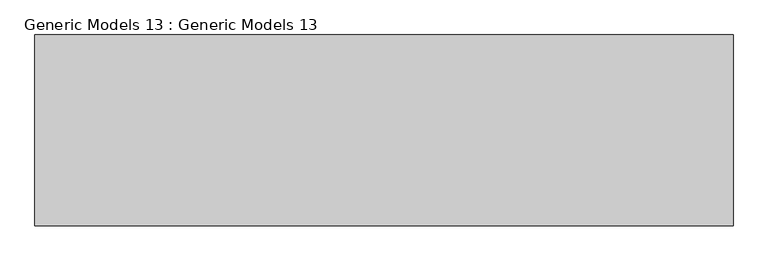
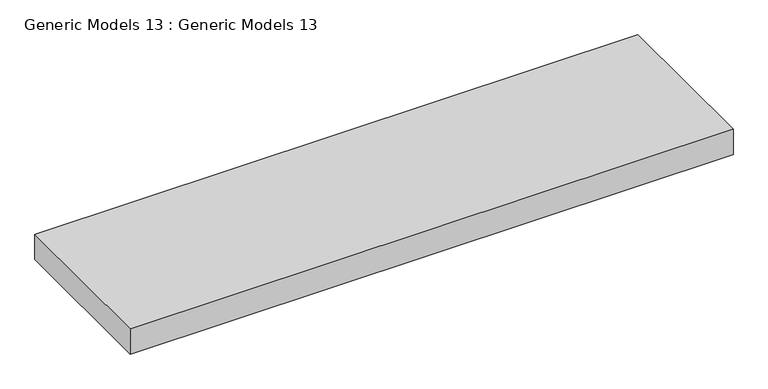
"""IFC4 building model written with IfcOpenShell, lengths in millimetres: proxy geometry, Generic Models 13 : Generic Models 13."""

from ifc_helpers import new_model, si_unit, frame, origin, place, context, project, spatial, polyline, outline, extrude, source, transform, mapped, element, save


def generic_models_13_generic_models_13_31af3d75(model_context):
    return source(origin(), model_context, "Body", "SweptSolid", [
        extrude(outline(polyline([(-16855.035389, 792.9828688), (-16855.035389, 1730.8186766), (-13425.5161422, 1730.8186766), (-13425.5161422, 792.9828688), (-16855.035389, 792.9828688)])), frame((0.0, 0.0, 5544.590558), z_axis=(0.0, 0.0, 1.0), x_axis=(1.0, 0.0, 0.0)), (0.0, 0.0, 1.0), 152.4),
    ])


if __name__ == "__main__":
    model = new_model("IFC4")
    model_context = context("Model", 3, world=origin())
    ifc_project = project(units=[si_unit("LENGTHUNIT", "METRE", prefix="MILLI")], contexts=[model_context])
    site = spatial("IfcSite", under=ifc_project)
    building = spatial("IfcBuilding", under=site)
    placement = place(None, origin())
    generic_models_13_generic_models_13_shape = generic_models_13_generic_models_13_31af3d75(model_context)
    element("IfcBuildingElementProxy", 1, Name="Generic Models 13 : Generic Models 13", ObjectType="Generic Models 13 : Generic Models 13", at=placement, inside=building, context=model_context, shape_type="MappedRepresentation", body=[
        mapped(generic_models_13_generic_models_13_shape, transform((0.0, 0.0, 0.0), x_axis=(1.0, 0.0, 0.0), y_axis=(0.0, 1.0, 0.0), z_axis=(0.0, 0.0, 1.0))),
    ])
    save(model, "model.ifc")
